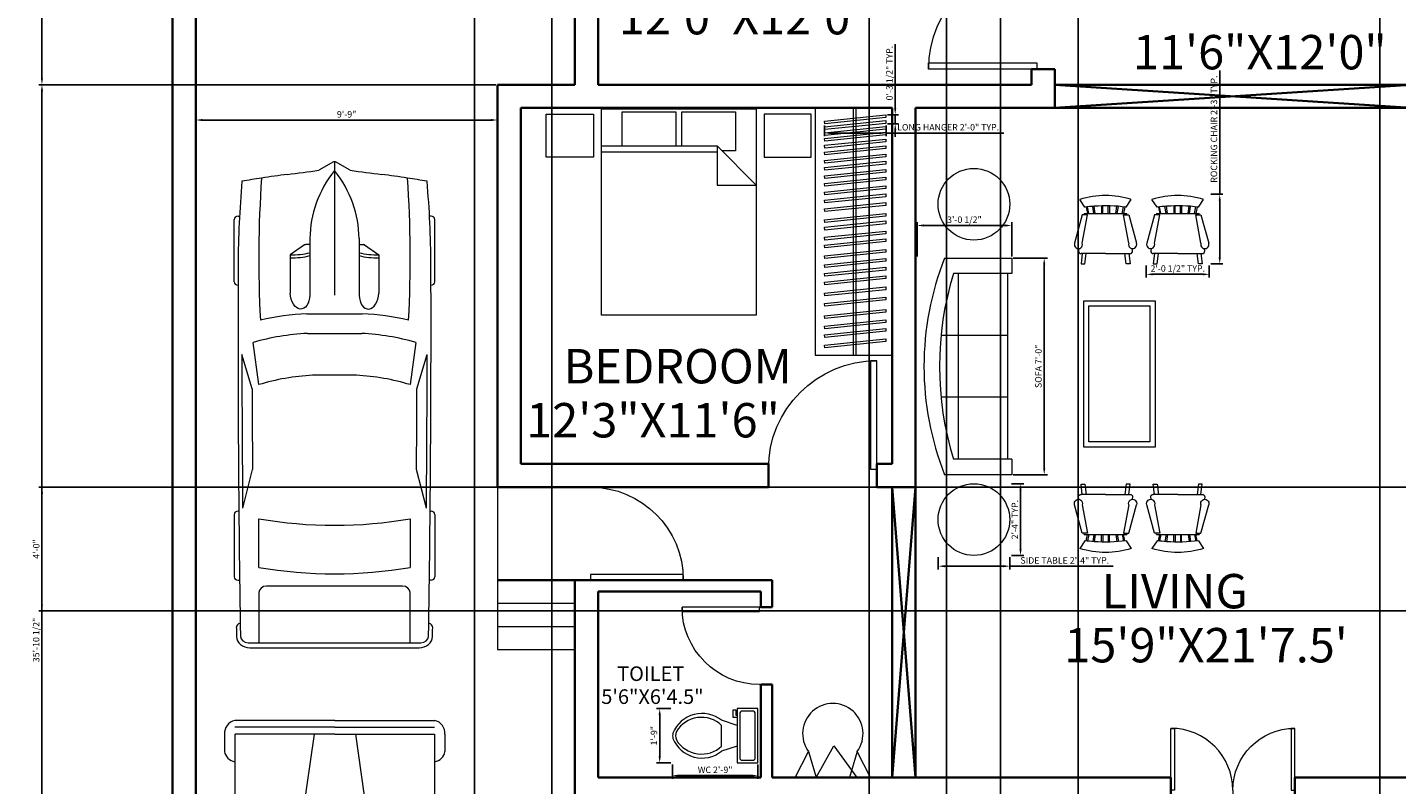
# Model space of a CAD drawing. Units: inches. Extents: x 3412 to 4225, y 13529 to 14581.
# Tile 3 of 7: x 3412 to 3943, y 13928 to 14222. Entities that reach past the tile are written whole.
import ezdxf

# ---------------------------------------------------------------- set-up
doc = ezdxf.new("R2010")
doc.units = ezdxf.units.IN
for name, color, linetype, lineweight in [('A-ANNO-DIMS', 2, 'Continuous', 13), ('A-AREA-IDEN', 7, 'Continuous', 18), ('A-DOOR', 4, 'Continuous', 18), ('A-FLOR-CASE', 9, 'Continuous', 18), ('A-FLOR-FIXT', 8, 'Continuous', 18), ('A-FLOR-STRS', 3, 'Continuous', 18), ('A-FURN', 8, 'Continuous', 18), ('A-WALL', 7, 'Continuous', 35), ('C-PKNG-VEHI', 8, 'Continuous', 13), ('C-SITE-WALL', 7, 'Continuous', 35)]:
    doc.layers.add(name, color=color, linetype=linetype, lineweight=lineweight)
doc.styles.get("Standard").update_dxf_attribs({"font": 'arial.ttf'})
doc.dimstyles.new('ISO-25', dxfattribs={"dimtxt": 2.5, "dimasz": 2.5, "dimexe": 1.25, "dimexo": 0.625, "dimtad": 1, "dimdec": 0, "dimlunit": 3, "dimtxsty": 'Standard', "dimcen": 2.5, "dimadec": 0, "dimazin": 0, "dimtfac": 1, "dimtdec": 0, "dimtmove": 0, "dimatfit": 3, "dimfxl": 1, "dimarcsym": 0})

# ---------------------------------------------------------------- blocks, each defined once
blk = doc.blocks.new('*U3')
for p, q in [((0, 0), (0, -5)), ((30, 0), (30, -5))]:
    blk.add_line(p, q)
blk.add_lwpolyline([(0, 0), (0, 30), (1.75, 30), (1.75, 0)], close=True)
blk.add_arc((0, 0), 30, 0, 90)
blk = doc.blocks.new('Toilet - top')
for p, q in [((9.5, -6), (9.5, -2)), ((-10, -8.5), (-8, -8.5)), ((-10, -9.5), (-10, -8.5)), ((-7, -9.5), (-10, -9.5)), ((-8, -8.5), (-8, -8)), ((-7, -8), (-7, -9.5)), ((-4, -8), (-6, -14)), ((4, -8), (6, -14)), ((4, -14), (-4, -14))]:
    blk.add_line(p, q)
blk.add_lwpolyline([(10.5, -8), (10.5, 0), (-10.5, 0), (-10.5, -8)], close=True)
for points in [[(-9.5, -2), (-9.5, -6)], [(8.5, -1), (-8.5, -1)], [(-8.5, -7), (8.5, -7)]]:
    blk.add_lwpolyline(points)
for centre, radius, start, end in [((-8.62, -1.88), 0.884, 81.8699, 188.1301), ((8.62, -1.88), 0.884, 351.8699, 98.1301), ((-8.62, -6.12), 0.884, 171.8699, 278.1301), ((8.62, -6.12), 0.884, 261.8699, 8.1301), ((3.52, -21.58), 12.17, 141.4691, 247.9714), ((4.2, -21.82), 11.33, 136.3677, 238.9468), ((-3.52, -21.58), 12.17, 292.0284, 38.5307), ((-4.2, -21.82), 11.33, 301.053, 43.6321), ((0, -27.88), 4, 245.7318, 294.2682), ((0, -29), 4, 254.8605, 285.1395)]:
    blk.add_arc(centre, radius, start, end)
blk = doc.blocks.new('Bed - Queen')
for p, q in [((0, -80.00003), (0, 0)), ((0, 0), (59.99999, 0)), ((59.99999, 0), (59.99999, -80.00003)), ((7.99999, -1.2), (28.79998, -1.2)), ((7.99999, -14.4), (7.99999, -1.2)), ((28.79998, -1.2), (28.79998, -14.4)), ((31.19999, -1.2), (51.99999, -1.2)), ((31.19999, -14.4), (31.19999, -1.2)), ((51.99999, -1.2), (51.99999, -16.4)), ((0, -14.4), (44.8, -14.4)), ((59.99999, -29.6), (44.8, -14.4)), ((44.8, -14.4), (44.8, -29.6)), ((44.8, -16.8), (0, -16.8)), ((51.99999, -16.4), (46.79936, -16.4)), ((44.8, -29.6), (59.99999, -29.6)), ((59.99999, -80.00003), (0, -80.00003))]:
    blk.add_line(p, q)
blk = doc.blocks.new('Sofa - Roundback 7 ft.')
for p, q in [((-12.00002, -32.4421), (-12.00003, -6.5971)), ((11.99997, -32.4421), (11.99998, -6.5971)), ((-36.000027, -34), (-36.000027, -11.4696)), ((-35.999844, -13.3819), (35.9998, -13.3819)), ((35.99998, -34), (35.99998, -11.4696)), ((-36.000027, -32.4421), (35.99998, -32.4421))]:
    blk.add_line(p, q)
for points in [[(-36.000027, -34), (-42.000027, -34), (-42.000027, -8)], [(41.99998, -8), (41.99998, -34), (35.99998, -34)]]:
    blk.add_lwpolyline(points)
for centre, radius, start, end in [((0, -114.25), 114.25, 68.43141, 111.5686), ((-0.00001, -127.1968), 121.1968, 72.72033, 107.2797)]:
    blk.add_arc(centre, radius, start, end)
blk = doc.blocks.new('Chair - Rocking')
for p, q in [((-8, -4.5), (-10, -1.5)), ((-7.5, -4.5), (-7, -7)), ((-6.5, -7), (-7.02225, -4.43)), ((-4.5, -7), (-4.96674, -4.19951)), ((-4, -7), (-4.40532, -4.16272)), ((-1.5, -4.05012), (-1.5, -7)), ((-1, -7), (-1, -4.05012)), ((1, -7), (1, -4.04655)), ((1.5, -4.05012), (1.5, -7)), ((4, -7), (4.40187, -4.18694)), ((4.5, -7), (4.96761, -4.19437)), ((6.5, -7), (7, -4.4057)), ((7.5, -4.5), (7, -7)), ((8, -4.5), (10, -1.5)), ((-9, -7.5), (-12, -18.49999)), ((-7, -7.5), (-9, -7.5)), ((-9, -18.49999), (-7, -7.5)), ((-8.23428, -6.99939), (-8.3093, -7.47958)), ((-8.23041, -7), (8.23915, -7)), ((7, -7.5), (9, -7.5)), ((9, -18.49999), (7, -7.5)), ((8.31071, -7.48854), (8.23449, -7.00073)), ((9, -7.5), (12, -18.49999)), ((-10.36644, -20.64523), (-10.5, -21.49999)), ((10.5, -21.49999), (10.3575, -20.58798)), ((-9, -22.49999), (-9.5, -26.49999)), ((0, -22.49999), (-9.5, -22.49999)), ((-9.5, -26.49999), (-8, -26.49999)), ((-8, -26.49999), (-7.5, -22.49999)), ((0, -22.49999), (9.5, -22.49999)), ((8, -26.49999), (7.5, -22.49999)), ((9.5, -26.49999), (8, -26.49999)), ((9, -22.49999), (9.5, -26.49999))]:
    blk.add_line(p, q)
for centre, radius, start, end in [((0, -34.08333), 34.08333, 72.93847, 107.0615), ((0, -68.25004), 64.25, 93.92211, 97.15267), ((0, -68.25004), 64.25, 82.84733, 93.92211), ((-10.5, -18.99999), 1.58114, 161.5651, 18.43495), ((10.5, -18.99999), 1.58114, 161.5651, 18.43495), ((-9.5, -21.49999), 1, 180, 270), ((9.5, -21.49999), 1, 270, 0)]:
    blk.add_arc(centre, radius, start, end)
blk = doc.blocks.new('*U19')
for p, q in [((21.1, 37.41), (21.1, 36.83)), ((46.55, 38.89), (22.35, 38.89)), ((47.8, 37.39), (47.8, 37.41)), ((135.45, 37.07), (135.45, 37.41)), ((136.7, 38.89), (160.9, 38.89)), ((162.15, 37.41), (162.15, 36.77)), ((87.99, 31.87), (74.76, 35.92)), ((134.31, 35.6), (119.29, 31.78)), ((186.47, -33.5), (186.47, 33.5)), ((188.4, -32.76), (188.4, 32.76)), ((70.03, 31.54), (86.41, 29.35)), ((138.42, 29.35), (157.25, 29.35)), ((186.47, 29.35), (167.01, 29.35)), ((164.52, 26.39), (164.52, -26.39)), ((32.27, 11.63), (36.13, 17.17)), ((36.13, 17.17), (50.94, 17.17)), ((32.12, 9.51), (32.12, 11.15)), ((58.92, -10.77), (58.92, 10.77)), ((3.27, 6.13), (0.1, 0.41)), ((29.77, 9.51), (51.68, 9.51)), ((66.55, -10.53), (66.55, 10.53)), ((82.74, 8.5), (82.74, -8.5)), ((186.47, -10.53), (186.47, 10.53)), ((0, 0), (51.68, 0)), ((0.1, -0.41), (3.27, -6.13)), ((29.77, -9.51), (51.68, -9.51)), ((32.12, -9.51), (32.12, -11.15)), ((32.27, -11.63), (36.13, -17.17)), ((36.13, -17.17), (50.94, -17.17)), ((86.41, -29.35), (70.03, -31.54)), ((134.31, -35.6), (119.29, -31.78)), ((157.25, -29.35), (138.42, -29.35)), ((167.01, -29.35), (186.47, -29.35)), ((21.1, -37.41), (21.1, -36.83)), ((87.99, -31.87), (74.76, -35.92)), ((135.45, -37.07), (135.45, -37.41)), ((162.15, -37.41), (162.15, -36.77)), ((46.55, -38.89), (22.35, -38.89)), ((47.8, -37.39), (47.8, -37.41)), ((136.7, -38.89), (160.9, -38.89))]:
    blk.add_line(p, q)
for centre, major_axis, ratio, start_param, end_param in [((41.19, -490.86), (0, 528.23), 0.842304, 0.00281, 0.075598), ((22.35, 37.41), (0, -1.48), 0.842304, 3.141593, 4.712389), ((64.48, -10555.62), (0, 10593.03), 0.842304, -0.013397, 0.002797), ((46.55, 37.41), (0, 1.48), 0.842304, -1.570796, 0), ((136.7, 37.41), (0, -1.48), 0.842304, 3.141593, 4.712389), ((160.9, 37.41), (0, 1.48), 0.842304, -1.570796, 0), ((180.63, 35.84), (0, 2.22), 0.842304, -0.013017, 1.249894), ((64.48, -10556.36), (0, 10595.31), 0.842304, -0.013397, -0.013017), ((183.98, 32.76), (0, -5.25), 0.842304, 1.570796, 3.128196), ((266.03, -27.52), (0, 313.31), 0.842304, 1.367076, 1.39176), ((64.48, -10555.62), (0, -10591.55), 0.842304, 3.133765, 3.140441), ((95.79, -3666.35), (0, -3698.24), 0.842304, 3.134049, 3.144098), ((183.98, 33.5), (0, -2.96), 0.842304, 1.570796, 3.128196), ((259.18, -27.52), (0, -305.3), 0.842304, 4.528606, 4.561838), ((37.47, -593.96), (0, -623.33), 0.842304, 3.096046, 3.200911), ((134.4, 5.39), (0, -89.78), 0.842304, 4.449482, 4.652344), ((135.29, 5.39), (0, 81.77), 0.842304, 1.245306, 1.50788), ((149.6, 2.8), (0, -79.58), 0.842304, 4.372215, 4.640744), ((17.08, 0), (0, 147.02), 0.842304, 4.511394, 4.913384), ((35.91, 0), (0, 147.02), 0.842304, 4.511394, 4.913384), ((167.01, 26.39), (0, 2.96), 0.842304, 0, 1.570796), ((-204.49, 52.4), (0, -250.96), 0.842304, 1.385369, 1.434372), ((13.04, 17.01), (0, 27.42), 0.842304, 4.435146, 4.718221), ((14.2, 17.01), (0, 27.42), 0.842304, 4.435146, 4.718221), ((50.79, 13.34), (6.34, -0.36), 0.603834, -1.395552, 1.581315), ((32.75, 11.15), (0, 0.74), 0.842304, 0.879714, 1.570796), ((29.77, -46.66), (0, 56.17), 0.842304, 0, 0.590319), ((0.62, 0), (0, -0.74), 0.842304, 4.131459, 5.293319), ((29.77, 46.66), (0, 56.17), 0.842304, 2.551274, 3.141593), ((-204.49, -52.4), (0, 250.96), 0.842304, -1.434372, -1.385369), ((13.04, -17.01), (0, -27.42), 0.842304, 1.564964, 1.848039), ((14.2, -17.01), (0, -27.42), 0.842304, 1.564964, 1.848039), ((135.29, -5.39), (0, -81.77), 0.842304, -1.50788, -1.245306), ((149.6, -2.8), (0, -79.58), 0.842304, -1.499151, -1.230623), ((32.75, -11.15), (0, -0.74), 0.842304, 4.712389, 5.403472), ((134.4, -5.39), (0, -89.78), 0.842304, -1.510751, -1.307889), ((259.18, 27.52), (0, 305.3), 0.842304, 1.721348, 1.754579), ((167.01, -26.39), (0, -2.96), 0.842304, 4.712389, 6.283185), ((266.03, 27.52), (0, 313.31), 0.842304, 1.749832, 1.774517), ((37.47, 593.96), (0, -623.33), 0.842304, -0.059319, 0.045547), ((95.79, 3666.35), (0, -3698.24), 0.842304, -0.002505, 0.007544), ((41.19, 490.86), (0, -528.23), 0.842304, -0.075598, -0.00281), ((64.48, 10555.62), (0, 10593.03), 0.842304, 3.138796, 3.15499), ((64.48, 10555.62), (0, -10591.55), 0.842304, 0.001152, 0.007828), ((180.63, -35.84), (0, -2.22), 0.842304, -1.249894, 0.013017), ((183.98, -33.5), (0, 2.96), 0.842304, 3.15499, 4.712389), ((183.98, -32.76), (0, -5.25), 0.842304, 0.013397, 1.570796), ((22.35, -37.41), (0, 1.48), 0.842304, 1.570796, 3.141593), ((46.55, -37.41), (0, -1.48), 0.842304, 0, 1.570796), ((136.7, -37.41), (0, -1.48), 0.842304, -1.570796, 0), ((160.9, -37.41), (0, 1.48), 0.842304, 3.141593, 4.712389), ((64.48, 10556.36), (0, 10595.31), 0.842304, 3.15461, 3.15499)]:
    blk.add_ellipse(centre, major_axis=major_axis, ratio=ratio, start_param=start_param, end_param=end_param)
at = {"extrusion": (0, 0, -1)}
blk.add_ellipse((50.79, -13.34), major_axis=(6.34, 0.36), ratio=0.603834, start_param=-1.395552, end_param=1.581315, dxfattribs=at)
blk = doc.blocks.new('*U20')
for p, q in [((0.1, -0.41), (0.1, 38.35)), ((2.77, -0.41), (2.77, 38.31)), ((5.44, 42.31), (12.12, 42.31)), ((5.44, -0.41), (5.44, 38.24)), ((5.45, 38.31), (16.12, 38.31)), ((16.12, 38.31), (180.34, 38.31)), ((61.52, -0.41), (61.52, 38.31)), ((61.52, 38.31), (77.54, 27.62)), ((64.19, 38.31), (76.2, 30.29)), ((76.2, 30.29), (76.2, 38.31)), ((78.87, 38.31), (78.87, 28.96)), ((106.91, 28.96), (106.91, 38.31)), ((109.58, 27.62), (109.58, 38.31)), ((112.25, 38.31), (112.25, 28.96)), ((140.29, 28.96), (140.29, 38.31)), ((141.62, 27.62), (149.64, 38.31)), ((149.64, -0.41), (149.64, 38.31)), ((189.69, 38.31), (179.01, 38.31)), ((189.69, 42.31), (183.01, 42.31)), ((189.69, -0.41), (189.69, 38.24)), ((192.36, -0.41), (192.36, 38.31)), ((195.03, -0.41), (195.03, 38.35)), ((77.54, 27.62), (141.62, 27.62)), ((77.54, -0.41), (77.54, 27.62)), ((78.87, 28.96), (106.91, 28.96)), ((112.25, 28.96), (140.29, 28.96)), ((141.62, -0.41), (141.62, 27.62)), ((5.44, 7.6), (61.52, 15.61)), ((0.1, -0.42), (0.1, -39.18)), ((2.77, -0.41), (2.77, -39.13)), ((5.44, -0.42), (5.44, -39.07)), ((61.52, -0.41), (61.52, -39.13)), ((77.54, -0.41), (77.54, -28.45)), ((141.62, -0.41), (141.62, -28.45)), ((149.64, -0.41), (149.64, -39.13)), ((189.69, -0.42), (189.69, -39.07)), ((192.36, -0.41), (192.36, -39.13)), ((195.03, -0.42), (195.03, -39.18)), ((5.44, -8.42), (61.52, -16.43)), ((61.52, -39.13), (77.54, -28.45)), ((64.19, -39.13), (76.2, -31.12)), ((76.2, -31.12), (76.2, -39.13)), ((77.54, -28.45), (141.62, -28.45)), ((78.87, -39.13), (78.87, -29.79)), ((78.87, -29.79), (106.91, -29.79)), ((106.91, -29.79), (106.91, -39.13)), ((109.58, -28.45), (109.58, -39.13)), ((112.25, -29.79), (140.29, -29.79)), ((112.25, -39.13), (112.25, -29.79)), ((140.29, -29.79), (140.29, -39.13)), ((141.62, -28.45), (149.64, -39.13)), ((5.45, -39.13), (16.12, -39.13)), ((16.12, -39.13), (180.34, -39.13)), ((189.69, -39.13), (179.01, -39.13)), ((5.44, -43.14), (12.12, -43.14)), ((189.69, -43.14), (183.01, -43.14))]:
    blk.add_line(p, q)
for centre, radius, start, end in [((5.06, 37.26), 5.06, 85.6455, 168.0943), ((11.45, 37.64), 4.72, 8.1301, 81.87), ((183.68, 37.64), 4.72, 98.13, 171.8699), ((190.07, 37.26), 5.06, 11.9057, 94.3545), ((5.06, -38.09), 5.06, 191.9057, 274.3545), ((11.45, -38.46), 4.72, 278.13, 351.8699), ((183.68, -38.46), 4.72, 188.1301, 261.87), ((190.07, -38.09), 5.06, 265.6455, 348.0943)]:
    blk.add_arc(centre, radius, start, end)
blk = doc.blocks.new('*D22')
at = {"layer": 'A-ANNO-DIMS', "color": 0, "lineweight": -2, "transparency": 16777216}
for p, q in [((3477.36, 14198.81), (3477.36, 14184.49)), ((3594.36, 14198.81), (3594.36, 14184.49)), ((3591.86, 14185.74), (3479.86, 14185.74))]:
    blk.add_line(p, q, dxfattribs=at)
at = {"layer": 'A-ANNO-DIMS', "color": 0, "transparency": 16777216}
for points in [[(3479.86, 14186.16), (3479.86, 14185.33), (3477.36, 14185.74)], [(3591.86, 14186.16), (3591.86, 14185.33), (3594.36, 14185.74)]]:
    blk.add_solid(points, dxfattribs=at)
at = {"layer": 'Defpoints', "color": 0, "transparency": 16777216}
for p in [(3477.36, 14199.43), (3594.36, 14199.43), (3477.36, 14185.74)]:
    blk.add_point(p, dxfattribs=at)
at = {"layer": 'A-ANNO-DIMS', "color": 0, "transparency": 16777216, "insert": (3535.86, 14187.64), "char_height": 2.5, "attachment_point": 5}
blk.add_mtext('9\'-9"', dxfattribs=at)
blk = doc.blocks.new('NIGHTSTAND')
blk.add_lwpolyline([(0, 16.62), (18.31, 16.62), (18.31, 0), (0, 0)], close=True)
blk = doc.blocks.new('CLOSET-HANGER-LONG')
blk.add_lwpolyline([(0, 1.06), (23.72, 3.5), (23.82, 2.44), (0.11, 0)], close=True)
blk = doc.blocks.new('SIDE-TABLE-ROUND')
blk.add_circle((13.89, 13.89), 13.89)
blk = doc.blocks.new('*D38')
at = {"layer": 'A-ANNO-DIMS', "color": 0, "lineweight": -2, "transparency": 16777216}
for p, q in [((3874.29, 14156.98), (3874.29, 14204.94)), ((3870.86, 14156.98), (3875.54, 14156.98)), ((3874.29, 14132.48), (3874.29, 14154.48)), ((3870.86, 14129.98), (3875.54, 14129.98))]:
    blk.add_line(p, q, dxfattribs=at)
at = {"layer": 'A-ANNO-DIMS', "color": 0, "transparency": 16777216}
for points in [[(3873.87, 14154.48), (3874.7, 14154.48), (3874.29, 14156.98)], [(3873.87, 14132.48), (3874.7, 14132.48), (3874.29, 14129.98)]]:
    blk.add_solid(points, dxfattribs=at)
at = {"layer": 'Defpoints', "color": 0, "transparency": 16777216}
for p in [(3870.24, 14156.98), (3874.29, 14156.98), (3870.24, 14129.98)]:
    blk.add_point(p, dxfattribs=at)
at = {"layer": 'A-ANNO-DIMS', "color": 0, "transparency": 16777216, "insert": (3872.37, 14182.21), "char_height": 2.5, "attachment_point": 5, "rotation": 90}
blk.add_mtext('ROCKING CHAIR 2\'-3" TYP.', dxfattribs=at)
blk = doc.blocks.new('*D39')
at = {"layer": 'A-ANNO-DIMS', "color": 0, "lineweight": -2, "transparency": 16777216}
for p, q in [((3845.8, 14129.35), (3845.8, 14124.68)), ((3870.24, 14129.35), (3870.24, 14124.68)), ((3848.3, 14125.93), (3867.74, 14125.93))]:
    blk.add_line(p, q, dxfattribs=at)
at = {"layer": 'A-ANNO-DIMS', "color": 0, "transparency": 16777216}
for points in [[(3848.3, 14126.34), (3848.3, 14125.51), (3845.8, 14125.93)], [(3867.74, 14126.34), (3867.74, 14125.51), (3870.24, 14125.93)]]:
    blk.add_solid(points, dxfattribs=at)
at = {"layer": 'Defpoints', "color": 0, "transparency": 16777216}
for p in [(3845.8, 14129.98), (3870.24, 14129.98), (3870.24, 14125.93)]:
    blk.add_point(p, dxfattribs=at)
at = {"layer": 'A-ANNO-DIMS', "color": 0, "transparency": 16777216, "insert": (3858.02, 14127.85), "char_height": 2.5, "attachment_point": 5}
blk.add_mtext('2\'-0 1/2" TYP.', dxfattribs=at)
blk = doc.blocks.new('*D40')
at = {"layer": 'A-ANNO-DIMS', "color": 0, "lineweight": -2, "transparency": 16777216}
for p, q in [((3721.1, 14183.65), (3721.1, 14179.45)), ((3744.93, 14183.65), (3744.93, 14179.45)), ((3723.6, 14180.7), (3742.43, 14180.7)), ((3744.93, 14180.7), (3790.59, 14180.7))]:
    blk.add_line(p, q, dxfattribs=at)
at = {"layer": 'A-ANNO-DIMS', "color": 0, "transparency": 16777216}
for points in [[(3723.6, 14181.12), (3723.6, 14180.29), (3721.1, 14180.7)], [(3742.43, 14181.12), (3742.43, 14180.29), (3744.93, 14180.7)]]:
    blk.add_solid(points, dxfattribs=at)
at = {"layer": 'Defpoints', "color": 0, "transparency": 16777216}
for p in [(3721.1, 14184.28), (3744.93, 14184.28), (3744.93, 14180.7)]:
    blk.add_point(p, dxfattribs=at)
at = {"layer": 'A-ANNO-DIMS', "color": 0, "transparency": 16777216, "insert": (3769.01, 14182.62), "char_height": 2.5, "attachment_point": 5}
blk.add_mtext('LONG HANGER 2\'-0" TYP.', dxfattribs=at)
blk = doc.blocks.new('*D41')
at = {"layer": 'A-ANNO-DIMS', "color": 0, "lineweight": -2, "transparency": 16777216}
for p, q in [((3748.5, 14190.27), (3748.5, 14215.09)), ((3745.55, 14187.77), (3749.75, 14187.77)), ((3748.5, 14184.28), (3748.5, 14187.77)), ((3745.55, 14184.28), (3749.75, 14184.28)), ((3748.5, 14181.78), (3748.5, 14179.28))]:
    blk.add_line(p, q, dxfattribs=at)
at = {"layer": 'A-ANNO-DIMS', "color": 0, "transparency": 16777216}
for points in [[(3748.09, 14190.27), (3748.92, 14190.27), (3748.5, 14187.77)], [(3748.09, 14181.78), (3748.92, 14181.78), (3748.5, 14184.28)]]:
    blk.add_solid(points, dxfattribs=at)
at = {"layer": 'Defpoints', "color": 0, "transparency": 16777216}
for p in [(3744.93, 14187.77), (3748.5, 14187.77), (3744.93, 14184.28)]:
    blk.add_point(p, dxfattribs=at)
at = {"layer": 'A-ANNO-DIMS', "color": 0, "transparency": 16777216, "insert": (3746.58, 14203.93), "char_height": 2.5, "attachment_point": 5, "rotation": 90}
blk.add_mtext('0\'-3 1/2" TYP.', dxfattribs=at)
blk = doc.blocks.new('*D48')
at = {"layer": 'A-ANNO-DIMS', "color": 0, "lineweight": -2, "transparency": 16777216}
for p, q in [((3765.12, 14016.33), (3765.12, 14011.54)), ((3767.62, 14012.79), (3790.4, 14012.79)), ((3792.9, 14016.33), (3792.9, 14011.54)), ((3792.9, 14012.79), (3833.04, 14012.79))]:
    blk.add_line(p, q, dxfattribs=at)
at = {"layer": 'A-ANNO-DIMS', "color": 0, "transparency": 16777216}
for points in [[(3767.62, 14013.2), (3767.62, 14012.37), (3765.12, 14012.79)], [(3790.4, 14013.2), (3790.4, 14012.37), (3792.9, 14012.79)]]:
    blk.add_solid(points, dxfattribs=at)
at = {"layer": 'Defpoints', "color": 0, "transparency": 16777216}
for p in [(3765.12, 14016.95), (3792.9, 14016.95), (3792.9, 14012.79)]:
    blk.add_point(p, dxfattribs=at)
at = {"layer": 'A-ANNO-DIMS', "color": 0, "transparency": 16777216, "insert": (3814.22, 14014.7), "char_height": 2.5, "attachment_point": 5}
blk.add_mtext('SIDE TABLE 2\'-4" TYP.', dxfattribs=at)
blk = doc.blocks.new('*D49')
at = {"layer": 'A-ANNO-DIMS', "color": 0, "lineweight": -2, "transparency": 16777216}
for p, q in [((3793.53, 14044.73), (3798.32, 14044.73)), ((3797.07, 14019.45), (3797.07, 14042.23)), ((3793.53, 14016.95), (3798.32, 14016.95))]:
    blk.add_line(p, q, dxfattribs=at)
at = {"layer": 'A-ANNO-DIMS', "color": 0, "transparency": 16777216}
for points in [[(3796.65, 14042.23), (3797.49, 14042.23), (3797.07, 14044.73)], [(3796.65, 14019.45), (3797.49, 14019.45), (3797.07, 14016.95)]]:
    blk.add_solid(points, dxfattribs=at)
at = {"layer": 'Defpoints', "color": 0, "transparency": 16777216}
for p in [(3792.9, 14044.73), (3797.07, 14044.73), (3792.9, 14016.95)]:
    blk.add_point(p, dxfattribs=at)
at = {"layer": 'A-ANNO-DIMS', "color": 0, "transparency": 16777216, "insert": (3795.19, 14030.84), "char_height": 2.5, "attachment_point": 5, "rotation": 90}
blk.add_mtext('2\'-4" TYP.', dxfattribs=at)
blk = doc.blocks.new('*D50')
at = {"layer": 'A-ANNO-DIMS', "color": 0, "lineweight": -2, "transparency": 16777216}
for p, q in [((3794.28, 14132.26), (3807.5, 14132.26)), ((3806.25, 14050.76), (3806.25, 14129.76)), ((3794.28, 14048.26), (3807.5, 14048.26))]:
    blk.add_line(p, q, dxfattribs=at)
at = {"layer": 'A-ANNO-DIMS', "color": 0, "transparency": 16777216}
for points in [[(3805.84, 14129.76), (3806.67, 14129.76), (3806.25, 14132.26)], [(3805.84, 14050.76), (3806.67, 14050.76), (3806.25, 14048.26)]]:
    blk.add_solid(points, dxfattribs=at)
at = {"layer": 'Defpoints', "color": 0, "transparency": 16777216}
for p in [(3793.65, 14132.26), (3806.25, 14132.26), (3793.65, 14048.26)]:
    blk.add_point(p, dxfattribs=at)
at = {"layer": 'A-ANNO-DIMS', "color": 0, "transparency": 16777216, "insert": (3804.33, 14090.26), "char_height": 2.5, "attachment_point": 5, "rotation": 90}
blk.add_mtext('SOFA 7\'-0"', dxfattribs=at)
blk = doc.blocks.new('*D51')
at = {"layer": 'A-ANNO-DIMS', "color": 0, "lineweight": -2, "transparency": 16777216}
for p, q in [((3756.99, 14132.89), (3756.99, 14146.11)), ((3791.15, 14144.86), (3759.49, 14144.86)), ((3793.65, 14132.89), (3793.65, 14146.11))]:
    blk.add_line(p, q, dxfattribs=at)
at = {"layer": 'A-ANNO-DIMS', "color": 0, "transparency": 16777216}
for points in [[(3759.49, 14145.28), (3759.49, 14144.45), (3756.99, 14144.86)], [(3791.15, 14145.28), (3791.15, 14144.45), (3793.65, 14144.86)]]:
    blk.add_solid(points, dxfattribs=at)
at = {"layer": 'Defpoints', "color": 0, "transparency": 16777216}
for p in [(3756.99, 14144.86), (3756.99, 14132.26), (3793.65, 14132.26)]:
    blk.add_point(p, dxfattribs=at)
at = {"layer": 'A-ANNO-DIMS', "color": 0, "transparency": 16777216, "insert": (3775.32, 14146.78), "char_height": 2.5, "attachment_point": 5}
blk.add_mtext('3\'-0 1/2"', dxfattribs=at)
blk = doc.blocks.new('*D54')
at = {"layer": 'A-ANNO-DIMS', "color": 0, "lineweight": -2, "transparency": 16777216}
for p, q in [((3662.16, 13935.94), (3662.16, 13930.36)), ((3695.21, 13935.94), (3695.21, 13930.36)), ((3664.66, 13931.61), (3692.71, 13931.61))]:
    blk.add_line(p, q, dxfattribs=at)
at = {"layer": 'A-ANNO-DIMS', "color": 0, "transparency": 16777216}
for points in [[(3664.66, 13932.03), (3664.66, 13931.19), (3662.16, 13931.61)], [(3692.71, 13932.03), (3692.71, 13931.19), (3695.21, 13931.61)]]:
    blk.add_solid(points, dxfattribs=at)
at = {"layer": 'Defpoints', "color": 0, "transparency": 16777216}
for p in [(3662.16, 13936.57), (3695.21, 13936.57), (3695.21, 13931.61)]:
    blk.add_point(p, dxfattribs=at)
at = {"layer": 'A-ANNO-DIMS', "color": 0, "transparency": 16777216, "insert": (3678.69, 13933.53), "char_height": 2.5, "attachment_point": 5}
blk.add_mtext('WC 2\'-9"', dxfattribs=at)
blk = doc.blocks.new('*D55')
at = {"layer": 'A-ANNO-DIMS', "color": 0, "lineweight": -2, "transparency": 16777216}
for p, q in [((3661.54, 13957.57), (3655.96, 13957.57)), ((3657.21, 13955.07), (3657.21, 13939.07)), ((3661.54, 13936.57), (3655.96, 13936.57))]:
    blk.add_line(p, q, dxfattribs=at)
at = {"layer": 'A-ANNO-DIMS', "color": 0, "transparency": 16777216}
for points in [[(3656.79, 13955.07), (3657.62, 13955.07), (3657.21, 13957.57)], [(3656.79, 13939.07), (3657.62, 13939.07), (3657.21, 13936.57)]]:
    blk.add_solid(points, dxfattribs=at)
at = {"layer": 'Defpoints', "color": 0, "transparency": 16777216}
for p in [(3662.16, 13957.57), (3657.21, 13936.57), (3662.16, 13936.57)]:
    blk.add_point(p, dxfattribs=at)
at = {"layer": 'A-ANNO-DIMS', "color": 0, "transparency": 16777216, "insert": (3655.3, 13947.07), "char_height": 2.5, "attachment_point": 5, "rotation": 90}
blk.add_mtext('1\'-9"', dxfattribs=at)
blk = doc.blocks.new('*D61')
at = {"layer": 'A-ANNO-DIMS', "color": 0, "lineweight": -2, "transparency": 16777216}
for p, q in [((3477.36, 14408.81), (3477.36, 13550.58)), ((3585.36, 14408.81), (3585.36, 13550.58)), ((3479.86, 13551.83), (3582.86, 13551.83))]:
    blk.add_line(p, q, dxfattribs=at)
at = {"layer": 'A-ANNO-DIMS', "color": 0, "transparency": 16777216}
for points in [[(3479.86, 13552.25), (3479.86, 13551.42), (3477.36, 13551.83)], [(3582.86, 13552.25), (3582.86, 13551.42), (3585.36, 13551.83)]]:
    blk.add_solid(points, dxfattribs=at)
at = {"layer": 'Defpoints', "color": 0, "transparency": 16777216}
for p in [(3477.36, 14409.43), (3585.36, 14409.43), (3585.36, 13551.83)]:
    blk.add_point(p, dxfattribs=at)
at = {"layer": 'A-ANNO-DIMS', "color": 0, "transparency": 16777216, "insert": (3531.36, 13553.73), "char_height": 2.5, "attachment_point": 5}
blk.add_mtext('9\'-0"', dxfattribs=at)
blk = doc.blocks.new('*D62')
at = {"layer": 'A-ANNO-DIMS', "color": 0, "lineweight": -2, "transparency": 16777216}
for p, q in [((3585.36, 14408.81), (3585.36, 13550.58)), ((3615.36, 14408.81), (3615.36, 13550.58)), ((3587.86, 13551.83), (3612.86, 13551.83))]:
    blk.add_line(p, q, dxfattribs=at)
at = {"layer": 'A-ANNO-DIMS', "color": 0, "transparency": 16777216}
for points in [[(3587.86, 13552.25), (3587.86, 13551.42), (3585.36, 13551.83)], [(3612.86, 13552.25), (3612.86, 13551.42), (3615.36, 13551.83)]]:
    blk.add_solid(points, dxfattribs=at)
at = {"layer": 'Defpoints', "color": 0, "transparency": 16777216}
for p in [(3585.36, 14409.43), (3615.36, 14409.43), (3615.36, 13551.83)]:
    blk.add_point(p, dxfattribs=at)
at = {"layer": 'A-ANNO-DIMS', "color": 0, "transparency": 16777216, "insert": (3600.36, 13553.73), "char_height": 2.5, "attachment_point": 5}
blk.add_mtext('2\'-6"', dxfattribs=at)
blk = doc.blocks.new('*D63')
at = {"layer": 'A-ANNO-DIMS', "color": 0, "lineweight": -2, "transparency": 16777216}
for p, q in [((3615.36, 14408.81), (3615.36, 13550.58)), ((3738.36, 14408.81), (3738.36, 13550.58)), ((3617.86, 13551.83), (3735.86, 13551.83))]:
    blk.add_line(p, q, dxfattribs=at)
at = {"layer": 'A-ANNO-DIMS', "color": 0, "transparency": 16777216}
for points in [[(3617.86, 13552.25), (3617.86, 13551.42), (3615.36, 13551.83)], [(3735.86, 13552.25), (3735.86, 13551.42), (3738.36, 13551.83)]]:
    blk.add_solid(points, dxfattribs=at)
at = {"layer": 'Defpoints', "color": 0, "transparency": 16777216}
for p in [(3615.36, 14409.43), (3738.36, 14409.43), (3738.36, 13551.83)]:
    blk.add_point(p, dxfattribs=at)
at = {"layer": 'A-ANNO-DIMS', "color": 0, "transparency": 16777216, "insert": (3676.86, 13553.73), "char_height": 2.5, "attachment_point": 5}
blk.add_mtext('10\'-3"', dxfattribs=at)
blk = doc.blocks.new('*D64')
at = {"layer": 'A-ANNO-DIMS', "color": 0, "lineweight": -2, "transparency": 16777216}
for p, q in [((3738.36, 14408.81), (3738.36, 13550.58)), ((3768.36, 14408.81), (3768.36, 13550.58)), ((3740.86, 13551.83), (3765.86, 13551.83))]:
    blk.add_line(p, q, dxfattribs=at)
at = {"layer": 'A-ANNO-DIMS', "color": 0, "transparency": 16777216}
for points in [[(3740.86, 13552.25), (3740.86, 13551.42), (3738.36, 13551.83)], [(3765.86, 13552.25), (3765.86, 13551.42), (3768.36, 13551.83)]]:
    blk.add_solid(points, dxfattribs=at)
at = {"layer": 'Defpoints', "color": 0, "transparency": 16777216}
for p in [(3738.36, 14409.43), (3768.36, 14409.43), (3768.36, 13551.83)]:
    blk.add_point(p, dxfattribs=at)
at = {"layer": 'A-ANNO-DIMS', "color": 0, "transparency": 16777216, "insert": (3753.36, 13553.73), "char_height": 2.5, "attachment_point": 5}
blk.add_mtext('2\'-6"', dxfattribs=at)
blk = doc.blocks.new('*D65')
at = {"layer": 'A-ANNO-DIMS', "color": 0, "lineweight": -2, "transparency": 16777216}
for p, q in [((3768.36, 14408.81), (3768.36, 13550.58)), ((3789.36, 14408.81), (3789.36, 13550.58)), ((3770.86, 13551.83), (3786.86, 13551.83))]:
    blk.add_line(p, q, dxfattribs=at)
at = {"layer": 'A-ANNO-DIMS', "color": 0, "transparency": 16777216}
for points in [[(3770.86, 13552.25), (3770.86, 13551.42), (3768.36, 13551.83)], [(3786.86, 13552.25), (3786.86, 13551.42), (3789.36, 13551.83)]]:
    blk.add_solid(points, dxfattribs=at)
at = {"layer": 'Defpoints', "color": 0, "transparency": 16777216}
for p in [(3768.36, 14409.43), (3789.36, 14409.43), (3789.36, 13551.83)]:
    blk.add_point(p, dxfattribs=at)
at = {"layer": 'A-ANNO-DIMS', "color": 0, "transparency": 16777216, "insert": (3778.86, 13553.73), "char_height": 2.5, "attachment_point": 5}
blk.add_mtext('1\'-9"', dxfattribs=at)
blk = doc.blocks.new('*D66')
at = {"layer": 'A-ANNO-DIMS', "color": 0, "lineweight": -2, "transparency": 16777216}
for p, q in [((3789.36, 14408.81), (3789.36, 13550.58)), ((3819.36, 14408.81), (3819.36, 13550.58)), ((3791.86, 13551.83), (3816.86, 13551.83))]:
    blk.add_line(p, q, dxfattribs=at)
at = {"layer": 'A-ANNO-DIMS', "color": 0, "transparency": 16777216}
for points in [[(3791.86, 13552.25), (3791.86, 13551.42), (3789.36, 13551.83)], [(3816.86, 13552.25), (3816.86, 13551.42), (3819.36, 13551.83)]]:
    blk.add_solid(points, dxfattribs=at)
at = {"layer": 'Defpoints', "color": 0, "transparency": 16777216}
for p in [(3789.36, 14409.43), (3819.36, 14409.43), (3819.36, 13551.83)]:
    blk.add_point(p, dxfattribs=at)
at = {"layer": 'A-ANNO-DIMS', "color": 0, "transparency": 16777216, "insert": (3804.36, 13553.73), "char_height": 2.5, "attachment_point": 5}
blk.add_mtext('2\'-6"', dxfattribs=at)
blk = doc.blocks.new('*D67')
at = {"layer": 'A-ANNO-DIMS', "color": 0, "lineweight": -2, "transparency": 16777216}
for p, q in [((3819.36, 14408.81), (3819.36, 13550.58)), ((3936.36, 14408.81), (3936.36, 13550.58)), ((3821.86, 13551.83), (3933.86, 13551.83))]:
    blk.add_line(p, q, dxfattribs=at)
at = {"layer": 'A-ANNO-DIMS', "color": 0, "transparency": 16777216}
for points in [[(3821.86, 13552.25), (3821.86, 13551.42), (3819.36, 13551.83)], [(3933.86, 13552.25), (3933.86, 13551.42), (3936.36, 13551.83)]]:
    blk.add_solid(points, dxfattribs=at)
at = {"layer": 'Defpoints', "color": 0, "transparency": 16777216}
for p in [(3819.36, 14409.43), (3936.36, 14409.43), (3936.36, 13551.83)]:
    blk.add_point(p, dxfattribs=at)
at = {"layer": 'A-ANNO-DIMS', "color": 0, "transparency": 16777216, "insert": (3877.86, 13553.73), "char_height": 2.5, "attachment_point": 5}
blk.add_mtext('9\'-9"', dxfattribs=at)
blk = doc.blocks.new('*D73')
at = {"layer": 'A-ANNO-DIMS', "color": 0, "lineweight": -2, "transparency": 16777216}
for p, q in [((3623.73, 14352.43), (3416.51, 14352.43)), ((3417.76, 14349.93), (3417.76, 14201.93)), ((3593.73, 14199.43), (3416.51, 14199.43))]:
    blk.add_line(p, q, dxfattribs=at)
at = {"layer": 'A-ANNO-DIMS', "color": 0, "transparency": 16777216}
for points in [[(3417.34, 14349.93), (3418.17, 14349.93), (3417.76, 14352.43)], [(3417.34, 14201.93), (3418.17, 14201.93), (3417.76, 14199.43)]]:
    blk.add_solid(points, dxfattribs=at)
at = {"layer": 'Defpoints', "color": 0, "transparency": 16777216}
for p in [(3624.36, 14352.43), (3417.76, 14199.43), (3594.36, 14199.43)]:
    blk.add_point(p, dxfattribs=at)
at = {"layer": 'A-ANNO-DIMS', "color": 0, "transparency": 16777216, "insert": (3415.86, 14275.93), "char_height": 2.5, "attachment_point": 5, "rotation": 90}
blk.add_mtext('12\'-9"', dxfattribs=at)
blk = doc.blocks.new('*D74')
at = {"layer": 'A-ANNO-DIMS', "color": 0, "lineweight": -2, "transparency": 16777216}
for p, q in [((3593.73, 14199.43), (3416.51, 14199.43)), ((3417.76, 14196.93), (3417.76, 13771.43)), ((3623.73, 13768.93), (3416.51, 13768.93))]:
    blk.add_line(p, q, dxfattribs=at)
at = {"layer": 'A-ANNO-DIMS', "color": 0, "transparency": 16777216}
for points in [[(3417.34, 14196.93), (3418.17, 14196.93), (3417.76, 14199.43)], [(3417.34, 13771.43), (3418.17, 13771.43), (3417.76, 13768.93)]]:
    blk.add_solid(points, dxfattribs=at)
at = {"layer": 'Defpoints', "color": 0, "transparency": 16777216}
for p in [(3594.36, 14199.43), (3417.76, 13768.93), (3624.36, 13768.93)]:
    blk.add_point(p, dxfattribs=at)
at = {"layer": 'A-ANNO-DIMS', "color": 0, "transparency": 16777216, "insert": (3415.84, 13984.18), "char_height": 2.5, "attachment_point": 5, "rotation": 90}
blk.add_mtext('35\'-10 1/2"', dxfattribs=at)
blk = doc.blocks.new('*D85')
at = {"layer": 'A-ANNO-DIMS', "color": 0, "lineweight": -2, "transparency": 16777216}
for p, q in [((4007.73, 14043.43), (3416.51, 14043.43)), ((3417.76, 13997.93), (3417.76, 14040.93)), ((4007.73, 13995.43), (3416.51, 13995.43))]:
    blk.add_line(p, q, dxfattribs=at)
at = {"layer": 'A-ANNO-DIMS', "color": 0, "transparency": 16777216}
for points in [[(3417.34, 14040.93), (3418.17, 14040.93), (3417.76, 14043.43)], [(3417.34, 13997.93), (3418.17, 13997.93), (3417.76, 13995.43)]]:
    blk.add_solid(points, dxfattribs=at)
at = {"layer": 'Defpoints', "color": 0, "transparency": 16777216}
for p in [(3417.76, 14043.43), (4008.36, 14043.43), (4008.36, 13995.43)]:
    blk.add_point(p, dxfattribs=at)
at = {"layer": 'A-ANNO-DIMS', "color": 0, "transparency": 16777216, "insert": (3415.86, 14019.43), "char_height": 2.5, "attachment_point": 5, "rotation": 90}
blk.add_mtext('4\'-0"', dxfattribs=at)

msp = doc.modelspace()

# ---------------------------------------------------------------- linework, layer by layer
at = {"layer": 'A-FLOR-CASE'}
for p, q in [((3717.42, 14190.43), (3717.42, 14094.64)), ((3732.39, 14094.64), (3732.39, 14190.43)), ((3733.39, 14094.64), (3733.39, 14190.43)), ((3717.42, 14094.64), (3747.36, 14094.64))]:
    msp.add_line(p, q, dxfattribs=at)
at = {"layer": 'A-FLOR-FIXT'}
for p, q in [((3717.88, 13930.93), (3724.68, 13943.2)), ((3724.68, 13943.2), (3733.65, 13930.93)), ((3709.76, 13930.93), (3714.86, 13940.98)), ((3714.86, 13940.98), (3717.88, 13930.93)), ((3733.77, 13940.98), (3730.75, 13930.93)), ((3738.87, 13930.93), (3733.77, 13940.98))]:
    msp.add_line(p, q, dxfattribs=at)
msp.add_arc((3724.32, 13947.87), 11.7, 323.9226, 216.0774, dxfattribs=at)
at = {"layer": 'A-FLOR-STRS'}
for p, q in [((3594.36, 14043.43), (3594.36, 13980.43)), ((3594.36, 13998.43), (3624.36, 13998.43)), ((3594.36, 13989.43), (3624.36, 13989.43)), ((3594.36, 13980.43), (3624.36, 13980.43))]:
    msp.add_line(p, q, dxfattribs=at)
at = {"layer": 'A-FURN'}
for points in [[(3821.6, 14115.67), (3849.2, 14115.67), (3849.2, 14058.94), (3821.6, 14058.94)], [(3823.6, 14113.67), (3847.2, 14113.67), (3847.2, 14060.94), (3823.6, 14060.94)]]:
    msp.add_lwpolyline(points, close=True, dxfattribs=at)
at = {"layer": 'A-WALL'}
for p, q in [((3624.36, 14352.43), (3624.36, 14199.43)), ((3633.36, 14343.43), (3633.36, 14199.43)), ((3801.36, 14205.43), (3810.36, 14205.43)), ((3801.36, 14205.43), (3801.36, 14199.43)), ((3810.36, 14205.43), (3810.36, 14190.43)), ((3594.36, 14199.43), (3624.36, 14199.43)), ((3594.36, 14199.43), (3594.36, 14043.43)), ((3633.36, 14199.43), (3801.36, 14199.43)), ((3810.36, 14199.43), (3948.36, 14199.43)), ((3810.36, 14190.43), (3948.36, 14199.43)), ((3810.36, 14199.43), (3948.36, 14190.43)), ((3603.36, 14190.43), (3747.36, 14190.43)), ((3603.36, 14190.43), (3603.36, 14052.43)), ((3747.36, 14190.43), (3747.36, 14052.43)), ((3756.36, 14190.43), (3756.36, 14052.43)), ((3756.36, 14190.43), (3810.36, 14190.43)), ((3810.36, 14190.43), (3948.36, 14190.43)), ((3603.36, 14052.43), (3699.36, 14052.43)), ((3699.36, 14052.43), (3699.36, 14043.43)), ((3741.36, 14052.43), (3741.36, 14043.43)), ((3741.36, 14052.43), (3747.36, 14052.43)), ((3756.36, 14052.43), (3756.36, 13930.93)), ((3594.36, 14043.43), (3699.36, 14043.43)), ((3741.36, 14043.43), (3756.36, 14043.43)), ((3747.36, 14043.43), (3747.36, 13930.93)), ((3747.36, 14043.43), (3756.36, 13930.93)), ((3747.36, 13930.93), (3756.36, 14043.43)), ((3594.36, 14007.43), (3700.86, 14007.43)), ((3624.36, 14007.43), (3624.36, 13768.93)), ((3700.86, 14007.43), (3700.86, 13996.93)), ((3633.36, 14002.93), (3633.36, 13930.93)), ((3633.36, 14002.93), (3696.36, 14002.93)), ((3696.36, 14002.93), (3696.36, 13996.93)), ((3696.36, 13996.93), (3700.86, 13996.93)), ((3696.36, 13966.93), (3700.86, 13966.93)), ((3696.36, 13966.93), (3696.36, 13930.93)), ((3700.86, 13966.93), (3700.86, 13930.93)), ((3633.36, 13930.93), (3696.36, 13930.93)), ((3700.86, 13930.93), (3756.36, 13930.93)), ((3756.36, 13930.93), (3855.36, 13930.93)), ((3855.36, 13921.93), (3855.36, 13930.93)), ((3903.36, 13921.93), (3903.36, 13930.93)), ((3903.36, 13930.93), (3957.36, 13930.93))]:
    msp.add_line(p, q, dxfattribs=at)
at = {"layer": 'C-SITE-WALL'}
for p, q in [((3468.36, 14526.43), (3468.36, 13602.43)), ((3477.36, 14409.43), (3477.36, 13611.43))]:
    msp.add_line(p, q, dxfattribs=at)

# ---------------------------------------------------------------- block references
at = {"layer": 'A-DOOR'}
for p, xscale, yscale, zscale, rotation in [((3803.36, 14205.43), 1.399999999999999, 1.399999999999999, 1.399999999999999, 89.99999999999999), ((3630.36, 14007.43), -1.20000000000006, 1.20000000000006, 1.20000000000006, 270)]:
    msp.add_blockref('*U3', p, dxfattribs=dict(at, xscale=xscale, yscale=yscale, zscale=zscale, rotation=rotation))
for p, xscale, yscale, zscale in [((3741.36, 14050.43), -1.399999999999999, 1.399999999999999, 1.399999999999999), ((3855.36, 13925.93), 0.8, 0.8, 0.8), ((3903.36, 13925.93), -0.8, 0.8, 0.8)]:
    msp.add_blockref('*U3', p, dxfattribs=dict(at, xscale=xscale, yscale=yscale, zscale=zscale))
at = {"layer": 'A-DOOR', "xscale": -1, "rotation": 90}
msp.add_blockref('*U3', (3695.86, 13996.93), dxfattribs=at)
at = {"layer": 'A-FLOR-CASE'}
for p in [(3721.1, 14184.28), (3721.1, 14182.01), (3721.1, 14179.76), (3721.1, 14177.51), (3721.1, 14174.89), (3721.1, 14172.21), (3721.1, 14169.05), (3721.1, 14166.25), (3721.1, 14163.08), (3721.1, 14160.1), (3721.1, 14156.75), (3721.1, 14153.59), (3721.1, 14150.23), (3721.1, 14146.04), (3721.1, 14143.11), (3721.1, 14139.22), (3721.1, 14136.24), (3721.1, 14132.03), (3721.1, 14128.57), (3721.1, 14125.16), (3721.1, 14121.86), (3721.1, 14117.54), (3721.1, 14113.58), (3721.1, 14108.84), (3721.1, 14104.81), (3721.1, 14101.41), (3721.1, 14097.46)]:
    msp.add_blockref('CLOSET-HANGER-LONG', p, dxfattribs=at)
at = {"layer": 'A-FLOR-FIXT', "rotation": 270}
msp.add_blockref('Toilet - top', (3695.21, 13947.07), dxfattribs=at)
at = {"layer": 'A-FURN'}
for name, p in [('NIGHTSTAND', (3613.26, 14171.35)), ('Bed - Queen', (3634.62, 14190.14)), ('SIDE-TABLE-ROUND', (3765.12, 14139.2)), ('Chair - Rocking', (3830.02, 14156.48)), ('Chair - Rocking', (3858.02, 14156.48)), ('SIDE-TABLE-ROUND', (3765.12, 14016.95))]:
    msp.add_blockref(name, p, dxfattribs=at)
at = {"layer": 'A-FURN', "extrusion": (0, 0, -1), "zscale": -1}
msp.add_blockref('NIGHTSTAND', (-3715.98, 14171.35), dxfattribs=at)
at = {"layer": 'A-FURN', "rotation": 90}
msp.add_blockref('Sofa - Roundback 7 ft.', (3759.65, 14090.26), dxfattribs=at)
at = {"layer": 'A-FURN', "xscale": -1, "rotation": 180}
for p in [(3830.02, 14018.13), (3858.02, 14018.13)]:
    msp.add_blockref('Chair - Rocking', p, dxfattribs=at)
at = {"layer": 'C-PKNG-VEHI', "rotation": 270}
for name, p in [('*U19', (3531.16, 14169.58)), ('*U20', (3531.67, 13953.1))]:
    msp.add_blockref(name, p, dxfattribs=at)

# ---------------------------------------------------------------- texts
at = {"layer": 'A-AREA-IDEN'}
for s, height, p in [('12\'0"X12\'0"', 13.3293, (3641.36, 14218.95)), ('11\'6"X12\'0"', 13.3293, (3840.68, 14205.38)), ('BEDROOM ', 13.329, (3619.95, 14083.64)), ('12\'3"X11\'6"', 13.3293, (3605.45, 14062.7)), ('LIVING ', 13.329, (3828.53, 13996.44)), ('15\'9"X21\'7.5\'', 13.3293, (3814.04, 13975.5)), ('TOILET', 5.666, (3640.73, 13968.29)), ('5\'6"X6\'4.5"', 5.6659, (3634.57, 13959.39))]:
    msp.add_text(s, height=height, dxfattribs=at).set_placement(p)

# ---------------------------------------------------------------- dimensions: what is measured, and where the dimension line sits
at = {"layer": 'A-ANNO-DIMS'}
for base, p1, p2, override, picture, middle in [((3585.36, 13551.83), (3477.36, 14409.43), (3585.36, 14409.43), {"dimdec": 1, "dimlfac": 1, "dimrnd": 0, "dimzin": 1, "dimdsep": 46, "dimlunit": 4, "dimfrac": 2}, '*D61', (3531.36, 13553.73)), ((3615.36, 13551.83), (3585.36, 14409.43), (3615.36, 14409.43), {"dimdec": 1, "dimlfac": 1, "dimrnd": 0, "dimzin": 1, "dimdsep": 46, "dimlunit": 4, "dimfrac": 2}, '*D62', (3600.36, 13553.73)), ((3738.36, 13551.83), (3615.36, 14409.43), (3738.36, 14409.43), {"dimdec": 1, "dimlfac": 1, "dimrnd": 0, "dimzin": 1, "dimdsep": 46, "dimlunit": 4, "dimfrac": 2}, '*D63', (3676.86, 13553.73)), ((3768.36, 13551.83), (3738.36, 14409.43), (3768.36, 14409.43), {"dimdec": 1, "dimlfac": 1, "dimrnd": 0, "dimzin": 1, "dimdsep": 46, "dimlunit": 4, "dimfrac": 2}, '*D64', (3753.36, 13553.73)), ((3789.36, 13551.83), (3768.36, 14409.43), (3789.36, 14409.43), {"dimdec": 1, "dimlfac": 1, "dimrnd": 0, "dimzin": 1, "dimdsep": 46, "dimlunit": 4, "dimfrac": 2}, '*D65', (3778.86, 13553.73)), ((3819.36, 13551.83), (3789.36, 14409.43), (3819.36, 14409.43), {"dimdec": 1, "dimlfac": 1, "dimrnd": 0, "dimzin": 1, "dimdsep": 46, "dimlunit": 4, "dimfrac": 2}, '*D66', (3804.36, 13553.73)), ((3936.36, 13551.83), (3819.36, 14409.43), (3936.36, 14409.43), {"dimdec": 1, "dimlfac": 1, "dimrnd": 0, "dimzin": 1, "dimdsep": 46, "dimlunit": 4, "dimfrac": 2}, '*D67', (3877.86, 13553.73)), ((3477.36, 14185.74), (3594.36, 14199.43), (3477.36, 14199.43), {"dimclrd": 0, "dimclre": 0, "dimclrt": 0}, '*D22', (3535.86, 14187.64))]:
    dim = msp.add_linear_dim(base=base, p1=p1, p2=p2, dimstyle='ISO-25', override=override, dxfattribs=at)
    dim.commit()
    dim.dimension.update_dxf_attribs({"geometry": picture, "text_midpoint": middle})
for base, p1, p2, angle, picture, middle in [((3417.76, 14199.43), (3624.36, 14352.43), (3594.36, 14199.43), 90, '*D73', (3415.86, 14275.93)), ((3417.76, 13768.93), (3594.36, 14199.43), (3624.36, 13768.93), 90, '*D74', (3415.84, 13984.18)), ((3756.99, 14144.86), (3793.65, 14132.26), (3756.99, 14132.26), 180, '*D51', (3775.32, 14146.78)), ((3417.76, 14043.43), (4008.36, 13995.43), (4008.36, 14043.43), 90, '*D85', (3415.86, 14019.43)), ((3657.21, 13936.57), (3662.16, 13957.57), (3662.16, 13936.57), 270, '*D55', (3655.3, 13947.07))]:
    dim = msp.add_linear_dim(base=base, p1=p1, p2=p2, angle=angle, dimstyle='ISO-25', override={"dimdec": 1, "dimlfac": 1, "dimrnd": 0, "dimzin": 1, "dimdsep": 46, "dimlunit": 4, "dimfrac": 2}, dxfattribs=at)
    dim.commit()
    dim.dimension.update_dxf_attribs({"geometry": picture, "text_midpoint": middle})
for base, p1, p2, text, picture, middle in [((3748.5, 14187.77), (3744.93, 14184.28), (3744.93, 14187.77), '<> TYP.', '*D41', (3746.58, 14203.93)), ((3874.29, 14156.98), (3870.24, 14129.98), (3870.24, 14156.98), 'ROCKING CHAIR <> TYP.', '*D38', (3872.37, 14182.21)), ((3806.25, 14132.26), (3793.65, 14048.26), (3793.65, 14132.26), 'SOFA <>', '*D50', (3804.33, 14090.26)), ((3797.07, 14044.73), (3792.9, 14016.95), (3792.9, 14044.73), '<> TYP.', '*D49', (3795.19, 14030.84))]:
    dim = msp.add_linear_dim(base=base, p1=p1, p2=p2, angle=90, text=text, dimstyle='ISO-25', override={"dimdec": 1, "dimlfac": 1, "dimrnd": 0, "dimzin": 1, "dimdsep": 46, "dimlunit": 4, "dimfrac": 2}, dxfattribs=at)
    dim.commit()
    dim.dimension.update_dxf_attribs({"geometry": picture, "text_midpoint": middle})
for base, p1, p2, text, picture, middle in [((3744.93, 14180.7), (3721.1, 14184.28), (3744.93, 14184.28), 'LONG HANGER <> TYP.', '*D40', (3769.01, 14182.62)), ((3870.24, 14125.93), (3845.8, 14129.98), (3870.24, 14129.98), '<> TYP.', '*D39', (3858.02, 14127.85)), ((3792.9, 14012.79), (3765.12, 14016.95), (3792.9, 14016.95), 'SIDE TABLE <> TYP.', '*D48', (3814.22, 14014.7)), ((3695.209, 13931.6093), (3662.1627, 13936.5663), (3695.209, 13936.5663), 'WC <>', '*D54', (3678.6858, 13933.5269))]:
    dim = msp.add_linear_dim(base=base, p1=p1, p2=p2, text=text, dimstyle='ISO-25', override={"dimdec": 1, "dimlfac": 1, "dimrnd": 0, "dimzin": 1, "dimdsep": 46, "dimlunit": 4, "dimfrac": 2}, dxfattribs=at)
    dim.commit()
    dim.dimension.update_dxf_attribs({"geometry": picture, "text_midpoint": middle})

doc.saveas('drawing.dxf')
